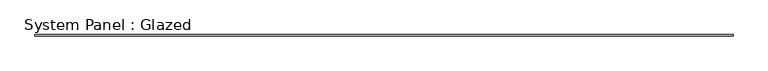
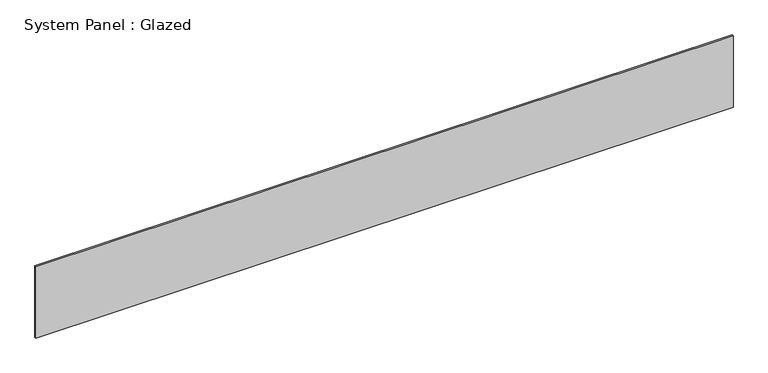
"""IFC4 building model written with IfcOpenShell, lengths in millimetres: plate geometry, System Panel : Glazed."""

from ifc_helpers import new_model, si_unit, origin, origin_with_axes, place, context, project, spatial, polyline, outline, extrude, source, transform, mapped, element, save


def system_panel_glazed_ea481271(model_context):
    return source(origin(), model_context, "Body", "SweptSolid", [
        extrude(outline(polyline([(5638.8, 19.05), (-5638.8, 19.05), (-5638.8, 44.45), (5638.8, 44.45), (5638.8, 19.05)])), origin_with_axes(), (0.0, 0.0, 1.0), 1219.2),
    ])


if __name__ == "__main__":
    model = new_model("IFC4")
    model_context = context("Model", 3, world=origin())
    ifc_project = project(units=[si_unit("LENGTHUNIT", "METRE", prefix="MILLI")], contexts=[model_context])
    site = spatial("IfcSite", under=ifc_project)
    building = spatial("IfcBuilding", under=site)
    placement = place(None, origin())
    system_panel_glazed_shape = system_panel_glazed_ea481271(model_context)
    element("IfcPlate", 1, ObjectType="System Panel : Glazed", at=placement, inside=building, context=model_context, shape_type="MappedRepresentation", body=[
        mapped(system_panel_glazed_shape, transform((0.0, 0.0, 0.0), x_axis=(1.0, 0.0, 0.0), y_axis=(0.0, 1.0, 0.0), z_axis=(0.0, 0.0, 1.0))),
    ])
    save(model, "model.ifc")

# Revit data of these elements
# Type "System Panel : Glazed"
#   Construction Type Id = "GSP4R"
#   Analytic Construction = "1/8 in Pilkington single glazing"
#   Visual Light Transmittance = 0.9
#   Solar Heat Gain Coefficient = 0.86
#   Heat Transfer Coefficient (U) = 1.18115 BTU/(h·ft²·°F)
# Element 1 (IfcPlate, "System Panel : Glazed")
#   Materials on its faces: "Glass"
# Materials
#   "Glass": class "Glass", colour RGB 0 128 192, transparency 0.75, Description = "Soda Lime Glass", Cost = 0
